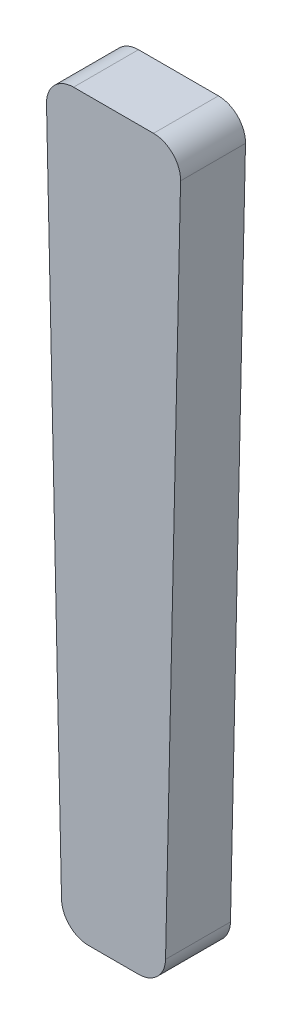
SolidWorks part; units mm, degrees
material "Plain Carbon Steel"
ref_plane "Front Plane" through (0, 0, 0) normal (0, 0, 1) x (1, 0, 0)
ref_plane "Top Plane" through (0, 0, 0) normal (0, 1, 0) x (1, 0, 0)
ref_plane "Right Plane" through (0, 0, 0) normal (1, 0, 0) x (0, 0, -1)
sketch "Cotter Profile Sketch" plane through (0, 0, 0) normal (0, 0, 1) x (1, 0, 0)
  line L0 (0, 88.0837) -> (0, -94.4093) construction
  line L1 (-7.3887, 77.0689) -> (7.3887, 77.0689)
  line L2 (12.3875, 71.9588) -> (9.6125, -54.0412)
  line L3 (4.6138, -58.9311) -> (-4.6138, -58.9311)
  line L4 (-9.6125, -54.0412) -> (-12.3875, 71.9588)
  arc A0 (7.3887, 77.0689) -> (12.3875, 71.9588) centre (7.3887, 72.0689) cw
  arc A1 (-7.3887, 77.0689) -> (-12.3875, 71.9588) centre (-7.3887, 72.0689) ccw
  arc A2 (4.6138, -58.9311) -> (9.6125, -54.0412) centre (4.6138, -53.9311) ccw
  arc A3 (-4.6138, -58.9311) -> (-9.6125, -54.0412) centre (-4.6138, -53.9311) cw
  point P9 (12.5, 77.0689)
  point P12 (-12.5, 77.0689)
  point P15 (9.5048, -58.9311)
  point P18 (-9.5048, -58.9311)
  point P19 (11, 8.9588)
  point P20 (-11, 8.9588)
  dimension "D6" = 5
  dimension "D7" = 5
  dimension "D1" = 136
  dimension "D2" = 25
  dimension "D3" = 22
  dimension "D4" = 12.5
  dimension "D5" = 11
  dimension "D8" = 77.0689
extrude "Cotter Body" add sketch "Cotter Profile Sketch" along normal mid plane 12
